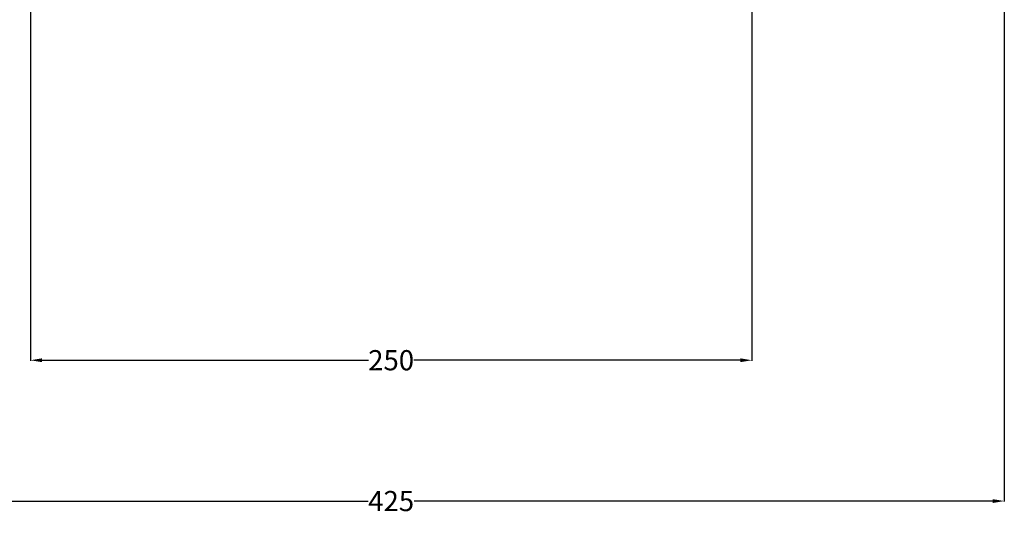
# Model space of a CAD drawing. Units: millimetres. Extents: x 0 to 2267, y 0 to 1823.
# Tile 23 of 256: x 1590 to 1931, y 902 to 1074. Entities that reach past the tile are written whole.
import ezdxf

# ---------------------------------------------------------------- set-up
doc = ezdxf.new("R2010")
doc.units = ezdxf.units.MM
doc.header["$MEASUREMENT"] = 0
doc.layers.add('M-DIMS', color=2, linetype='Continuous', lineweight=25)
doc.styles.get("Standard").update_dxf_attribs({"font": 'arial.ttf'})
doc.dimstyles.get("Standard").update_dxf_attribs({"dimtxt": 7, "dimasz": 4, "dimexe": 0.18, "dimexo": 0.0625, "dimgap": 0.09, "dimtad": 0, "dimdec": 0, "dimzin": 0, "dimdsep": 46, "dimtxsty": 'Standard', "dimcen": 0.09, "dimadec": 0, "dimazin": 0, "dimtfac": 1, "dimtdec": 0, "dimtofl": 0, "dimtmove": 0, "dimatfit": 3, "dimfxl": 1, "dimtolj": 1, "dimtzin": 0, "dimarcsym": 0})

# ---------------------------------------------------------------- blocks, each defined once
blk = doc.blocks.new('*D1')
at = {"layer": 'Defpoints', "color": 0, "transparency": 16777216}
for p in [(1593.43, 1127.42), (1843.43, 1127.42), (1843.43, 955.63)]:
    blk.add_point(p, dxfattribs=at)
at = {"layer": 'M-DIMS', "color": 0, "lineweight": -2, "transparency": 16777216}
for p, q in [((1593.43, 1127.35), (1593.43, 955.45)), ((1843.43, 1127.35), (1843.43, 955.45)), ((1597.43, 955.63), (1710.56, 955.63)), ((1839.43, 955.63), (1726.3, 955.63))]:
    blk.add_line(p, q, dxfattribs=at)
at = {"layer": 'M-DIMS', "color": 0, "transparency": 16777216}
for points in [[(1597.43, 956.29), (1597.43, 954.96), (1593.43, 955.63)], [(1839.43, 956.29), (1839.43, 954.96), (1843.43, 955.63)]]:
    blk.add_solid(points, dxfattribs=at)
at = {"layer": 'M-DIMS', "color": 0, "transparency": 16777216, "insert": (1718.43, 955.63), "char_height": 7, "attachment_point": 5}
blk.add_mtext('\\A1;250', dxfattribs=at)
blk = doc.blocks.new('*D2')
at = {"layer": 'Defpoints', "color": 0, "transparency": 16777216}
for p in [(1505.93, 1077.42), (1930.93, 1077.42), (1930.93, 906.79)]:
    blk.add_point(p, dxfattribs=at)
at = {"layer": 'M-DIMS', "color": 0, "lineweight": -2, "transparency": 16777216}
for p, q in [((1505.93, 1077.35), (1505.93, 906.61)), ((1930.93, 1077.35), (1930.93, 906.61)), ((1509.93, 906.79), (1710.44, 906.79)), ((1926.93, 906.79), (1726.42, 906.79))]:
    blk.add_line(p, q, dxfattribs=at)
at = {"layer": 'M-DIMS', "color": 0, "transparency": 16777216}
for points in [[(1509.93, 907.45), (1509.93, 906.12), (1505.93, 906.79)], [(1926.93, 907.45), (1926.93, 906.12), (1930.93, 906.79)]]:
    blk.add_solid(points, dxfattribs=at)
at = {"layer": 'M-DIMS', "color": 0, "transparency": 16777216, "insert": (1718.43, 906.79), "char_height": 7, "attachment_point": 5}
blk.add_mtext('\\A1;425', dxfattribs=at)

msp = doc.modelspace()

# ---------------------------------------------------------------- dimensions: what is measured, and where the dimension line sits
at = {"layer": 'M-DIMS'}
for base, p1, p2, picture, middle in [((1843.429, 955.628), (1593.429, 1127.417), (1843.429, 1127.417), '*D1', (1718.429, 955.628)), ((1930.929, 906.787), (1505.929, 1077.417), (1930.929, 1077.417), '*D2', (1718.429, 906.787))]:
    dim = msp.add_linear_dim(base=base, p1=p1, p2=p2, dimstyle='Standard', override={"dimclrd": 0, "dimclre": 0, "dimclrt": 0}, dxfattribs=at)
    dim.commit()
    dim.dimension.update_dxf_attribs({"geometry": picture, "text_midpoint": middle})

doc.saveas('drawing.dxf')
